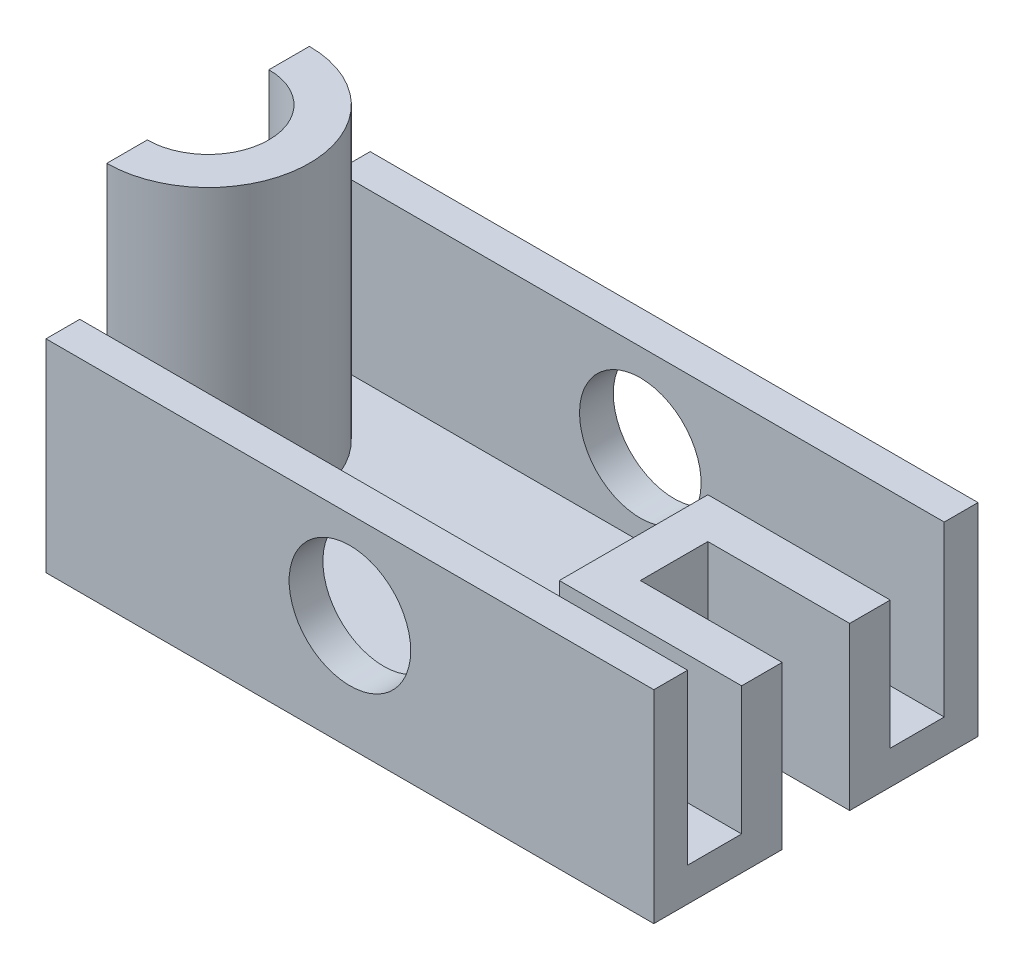
ISO-10303-21;
HEADER;
FILE_DESCRIPTION(('STEP AP214'),'2;1');
FILE_NAME('part.step','',(''),(''),'','','');
FILE_SCHEMA(('AUTOMOTIVE_DESIGN { 1 0 10303 214 1 1 1 1 }'));
ENDSEC;
DATA;
#1=APPLICATION_CONTEXT('core data for automotive mechanical design processes');
#2=APPLICATION_PROTOCOL_DEFINITION('international standard','automotive_design',2000,#1);
#3=PRODUCT_CONTEXT('',#1,'mechanical');
#4=PRODUCT('Part','Part','',(#3));
#5=PRODUCT_RELATED_PRODUCT_CATEGORY('part','',(#4));
#6=PRODUCT_DEFINITION_FORMATION('','',#4);
#7=PRODUCT_DEFINITION_CONTEXT('part definition',#1,'design');
#8=PRODUCT_DEFINITION('design','',#6,#7);
#9=PRODUCT_DEFINITION_SHAPE('','',#8);
#10=(LENGTH_UNIT() NAMED_UNIT(*) SI_UNIT(.MILLI.,.METRE.));
#11=(NAMED_UNIT(*) PLANE_ANGLE_UNIT() SI_UNIT($,.RADIAN.));
#12=(NAMED_UNIT(*) SI_UNIT($,.STERADIAN.) SOLID_ANGLE_UNIT());
#13=UNCERTAINTY_MEASURE_WITH_UNIT(LENGTH_MEASURE(1.E-05),#10,'distance_accuracy_value','');
#14=(GEOMETRIC_REPRESENTATION_CONTEXT(3) GLOBAL_UNCERTAINTY_ASSIGNED_CONTEXT((#13)) GLOBAL_UNIT_ASSIGNED_CONTEXT((#10,
#11,#12)) REPRESENTATION_CONTEXT('',''));
#15=CARTESIAN_POINT('',(0.,0.,0.));
#16=DIRECTION('',(0.,0.,1.));
#17=DIRECTION('',(1.,0.,0.));
#18=AXIS2_PLACEMENT_3D('',#15,#16,#17);
#19=CARTESIAN_POINT('',(45.,30.,24.));
#20=DIRECTION('',(-1.,0.,0.));
#21=DIRECTION('',(0.,0.,1.));
#22=AXIS2_PLACEMENT_3D('',#19,#20,#21);
#23=PLANE('',#22);
#24=DIRECTION('',(0.,0.,-1.));
#25=VECTOR('',#24,1.);
#26=CARTESIAN_POINT('',(45.,0.,24.));
#27=LINE('',#26,#25);
#28=CARTESIAN_POINT('',(45.,0.,24.));
#29=VERTEX_POINT('',#28);
#30=CARTESIAN_POINT('',(45.,0.,5.));
#31=VERTEX_POINT('',#30);
#32=EDGE_CURVE('E202',#29,#31,#27,.T.);
#33=ORIENTED_EDGE('',*,*,#32,.T.);
#34=DIRECTION('',(0.,1.,0.));
#35=VECTOR('',#34,1.);
#36=CARTESIAN_POINT('',(45.,0.,5.));
#37=LINE('',#36,#35);
#38=CARTESIAN_POINT('',(45.,24.,5.));
#39=VERTEX_POINT('',#38);
#40=EDGE_CURVE('E251',#31,#39,#37,.T.);
#41=ORIENTED_EDGE('',*,*,#40,.T.);
#42=DIRECTION('',(0.,0.,-1.));
#43=VECTOR('',#42,1.);
#44=CARTESIAN_POINT('',(45.,24.,-11.));
#45=LINE('',#44,#43);
#46=CARTESIAN_POINT('',(45.,24.,11.));
#47=VERTEX_POINT('',#46);
#48=EDGE_CURVE('E257',#47,#39,#45,.T.);
#49=ORIENTED_EDGE('',*,*,#48,.F.);
#50=DIRECTION('',(0.,-1.,0.));
#51=VECTOR('',#50,1.);
#52=CARTESIAN_POINT('',(45.,24.,11.));
#53=LINE('',#52,#51);
#54=CARTESIAN_POINT('',(45.,5.,11.));
#55=VERTEX_POINT('',#54);
#56=EDGE_CURVE('E267',#47,#55,#53,.T.);
#57=ORIENTED_EDGE('',*,*,#56,.T.);
#58=DIRECTION('',(0.,0.,1.));
#59=VECTOR('',#58,1.);
#60=CARTESIAN_POINT('',(45.,5.,-19.));
#61=LINE('',#60,#59);
#62=CARTESIAN_POINT('',(45.,5.,19.));
#63=VERTEX_POINT('',#62);
#64=EDGE_CURVE('E314',#55,#63,#61,.T.);
#65=ORIENTED_EDGE('',*,*,#64,.T.);
#66=DIRECTION('',(0.,1.,0.));
#67=VECTOR('',#66,1.);
#68=CARTESIAN_POINT('',(45.,30.,19.));
#69=LINE('',#68,#67);
#70=CARTESIAN_POINT('',(45.,30.,19.));
#71=VERTEX_POINT('',#70);
#72=EDGE_CURVE('E317',#63,#71,#69,.T.);
#73=ORIENTED_EDGE('',*,*,#72,.T.);
#74=DIRECTION('',(0.,0.,-1.));
#75=VECTOR('',#74,1.);
#76=CARTESIAN_POINT('',(45.,30.,24.));
#77=LINE('',#76,#75);
#78=CARTESIAN_POINT('',(45.,30.,24.));
#79=VERTEX_POINT('',#78);
#80=EDGE_CURVE('E333',#79,#71,#77,.T.);
#81=ORIENTED_EDGE('',*,*,#80,.F.);
#82=DIRECTION('',(0.,-1.,0.));
#83=VECTOR('',#82,1.);
#84=CARTESIAN_POINT('',(45.,30.,24.));
#85=LINE('',#84,#83);
#86=EDGE_CURVE('E224',#79,#29,#85,.T.);
#87=ORIENTED_EDGE('',*,*,#86,.T.);
#88=EDGE_LOOP('',(#33,#41,#49,#57,#65,#73,#81,#87));
#89=FACE_BOUND('',#88,.T.);
#90=ADVANCED_FACE('F43',(#89),#23,.F.);
#91=CARTESIAN_POINT('',(45.,5.,-19.));
#92=DIRECTION('',(0.,-1.,0.));
#93=DIRECTION('',(0.,0.,-1.));
#94=AXIS2_PLACEMENT_3D('',#91,#92,#93);
#95=PLANE('',#94);
#96=DIRECTION('',(-1.,0.,0.));
#97=VECTOR('',#96,1.);
#98=CARTESIAN_POINT('',(45.,5.,-11.));
#99=LINE('',#98,#97);
#100=CARTESIAN_POINT('',(45.,5.,-11.));
#101=VERTEX_POINT('',#100);
#102=CARTESIAN_POINT('',(18.,5.,-11.));
#103=VERTEX_POINT('',#102);
#104=EDGE_CURVE('E258',#101,#103,#99,.T.);
#105=ORIENTED_EDGE('',*,*,#104,.F.);
#106=CARTESIAN_POINT('',(45.,5.,-19.));
#107=VERTEX_POINT('',#106);
#108=EDGE_CURVE('E316',#107,#101,#61,.T.);
#109=ORIENTED_EDGE('',*,*,#108,.F.);
#110=DIRECTION('',(-1.,0.,0.));
#111=VECTOR('',#110,1.);
#112=CARTESIAN_POINT('',(45.,5.,-19.));
#113=LINE('',#112,#111);
#114=CARTESIAN_POINT('',(-45.,5.,-19.));
#115=VERTEX_POINT('',#114);
#116=EDGE_CURVE('E325',#107,#115,#113,.T.);
#117=ORIENTED_EDGE('',*,*,#116,.T.);
#118=DIRECTION('',(0.,0.,1.));
#119=VECTOR('',#118,1.);
#120=CARTESIAN_POINT('',(-45.,5.,-19.));
#121=LINE('',#120,#119);
#122=CARTESIAN_POINT('',(-45.,5.,-15.));
#123=VERTEX_POINT('',#122);
#124=EDGE_CURVE('E326',#115,#123,#121,.T.);
#125=ORIENTED_EDGE('',*,*,#124,.T.);
#126=CARTESIAN_POINT('',(-45.,5.,0.));
#127=DIRECTION('',(0.,-1.,0.));
#128=DIRECTION('',(0.,0.,-1.));
#129=AXIS2_PLACEMENT_3D('',#126,#127,#128);
#130=CIRCLE('',#129,15.);
#131=CARTESIAN_POINT('',(-45.,5.,15.));
#132=VERTEX_POINT('',#131);
#133=EDGE_CURVE('E11',#123,#132,#130,.T.);
#134=ORIENTED_EDGE('',*,*,#133,.T.);
#135=CARTESIAN_POINT('',(-45.,5.,19.));
#136=VERTEX_POINT('',#135);
#137=EDGE_CURVE('E324',#132,#136,#121,.T.);
#138=ORIENTED_EDGE('',*,*,#137,.T.);
#139=DIRECTION('',(-1.,0.,0.));
#140=VECTOR('',#139,1.);
#141=CARTESIAN_POINT('',(45.,5.,19.));
#142=LINE('',#141,#140);
#143=EDGE_CURVE('E332',#63,#136,#142,.T.);
#144=ORIENTED_EDGE('',*,*,#143,.F.);
#145=ORIENTED_EDGE('',*,*,#64,.F.);
#146=DIRECTION('',(1.,0.,0.));
#147=VECTOR('',#146,1.);
#148=CARTESIAN_POINT('',(45.,5.,11.));
#149=LINE('',#148,#147);
#150=CARTESIAN_POINT('',(18.,5.,11.));
#151=VERTEX_POINT('',#150);
#152=EDGE_CURVE('E275',#151,#55,#149,.T.);
#153=ORIENTED_EDGE('',*,*,#152,.F.);
#154=DIRECTION('',(0.,0.,1.));
#155=VECTOR('',#154,1.);
#156=CARTESIAN_POINT('',(18.,5.,-11.));
#157=LINE('',#156,#155);
#158=EDGE_CURVE('E66',#103,#151,#157,.T.);
#159=ORIENTED_EDGE('',*,*,#158,.F.);
#160=EDGE_LOOP('',(#105,#109,#117,#125,#134,#138,#144,#145,#153,#159));
#161=FACE_BOUND('',#160,.T.);
#162=ADVANCED_FACE('F368',(#161),#95,.F.);
#163=CARTESIAN_POINT('',(-45.,30.,24.));
#164=DIRECTION('',(1.,0.,0.));
#165=DIRECTION('',(0.,0.,-1.));
#166=AXIS2_PLACEMENT_3D('',#163,#164,#165);
#167=PLANE('',#166);
#168=DIRECTION('',(0.,0.,1.));
#169=VECTOR('',#168,1.);
#170=CARTESIAN_POINT('',(-45.,0.,24.));
#171=LINE('',#170,#169);
#172=CARTESIAN_POINT('',(-45.,0.,-24.));
#173=VERTEX_POINT('',#172);
#174=CARTESIAN_POINT('',(-45.,0.,-9.00000000000001));
#175=VERTEX_POINT('',#174);
#176=EDGE_CURVE('E220',#173,#175,#171,.T.);
#177=ORIENTED_EDGE('',*,*,#176,.T.);
#178=DIRECTION('',(0.,1.,0.));
#179=VECTOR('',#178,1.);
#180=CARTESIAN_POINT('',(-45.,0.,-9.00000000000001));
#181=LINE('',#180,#179);
#182=CARTESIAN_POINT('',(-45.,48.,-9.00000000000001));
#183=VERTEX_POINT('',#182);
#184=EDGE_CURVE('E294',#175,#183,#181,.T.);
#185=ORIENTED_EDGE('',*,*,#184,.T.);
#186=DIRECTION('',(0.,0.,-1.));
#187=VECTOR('',#186,1.);
#188=CARTESIAN_POINT('',(-45.,48.,15.));
#189=LINE('',#188,#187);
#190=CARTESIAN_POINT('',(-45.,48.,-15.));
#191=VERTEX_POINT('',#190);
#192=EDGE_CURVE('E300',#183,#191,#189,.T.);
#193=ORIENTED_EDGE('',*,*,#192,.T.);
#194=DIRECTION('',(0.,-1.,0.));
#195=VECTOR('',#194,1.);
#196=CARTESIAN_POINT('',(-45.,48.,-15.));
#197=LINE('',#196,#195);
#198=EDGE_CURVE('E304',#191,#123,#197,.T.);
#199=ORIENTED_EDGE('',*,*,#198,.T.);
#200=ORIENTED_EDGE('',*,*,#124,.F.);
#201=DIRECTION('',(0.,-1.,0.));
#202=VECTOR('',#201,1.);
#203=CARTESIAN_POINT('',(-45.,30.,-19.));
#204=LINE('',#203,#202);
#205=CARTESIAN_POINT('',(-45.,30.,-19.));
#206=VERTEX_POINT('',#205);
#207=EDGE_CURVE('E306',#206,#115,#204,.T.);
#208=ORIENTED_EDGE('',*,*,#207,.F.);
#209=DIRECTION('',(0.,0.,1.));
#210=VECTOR('',#209,1.);
#211=CARTESIAN_POINT('',(-45.,30.,24.));
#212=LINE('',#211,#210);
#213=CARTESIAN_POINT('',(-45.,30.,-24.));
#214=VERTEX_POINT('',#213);
#215=EDGE_CURVE('E340',#214,#206,#212,.T.);
#216=ORIENTED_EDGE('',*,*,#215,.F.);
#217=DIRECTION('',(0.,-1.,0.));
#218=VECTOR('',#217,1.);
#219=CARTESIAN_POINT('',(-45.,30.,-24.));
#220=LINE('',#219,#218);
#221=EDGE_CURVE('E228',#214,#173,#220,.T.);
#222=ORIENTED_EDGE('',*,*,#221,.T.);
#223=EDGE_LOOP('',(#177,#185,#193,#199,#200,#208,#216,#222));
#224=FACE_BOUND('',#223,.T.);
#225=ADVANCED_FACE('F409',(#224),#167,.F.);
#226=CARTESIAN_POINT('',(0.,30.,0.));
#227=DIRECTION('',(0.,-1.,0.));
#228=DIRECTION('',(0.,0.,-1.));
#229=AXIS2_PLACEMENT_3D('',#226,#227,#228);
#230=PLANE('',#229);
#231=ORIENTED_EDGE('',*,*,#215,.T.);
#232=DIRECTION('',(-1.,0.,0.));
#233=VECTOR('',#232,1.);
#234=CARTESIAN_POINT('',(45.,30.,-19.));
#235=LINE('',#234,#233);
#236=CARTESIAN_POINT('',(45.,30.,-19.));
#237=VERTEX_POINT('',#236);
#238=EDGE_CURVE('E206',#237,#206,#235,.T.);
#239=ORIENTED_EDGE('',*,*,#238,.F.);
#240=CARTESIAN_POINT('',(45.,30.,-24.));
#241=VERTEX_POINT('',#240);
#242=EDGE_CURVE('E225',#237,#241,#77,.T.);
#243=ORIENTED_EDGE('',*,*,#242,.T.);
#244=DIRECTION('',(-1.,0.,0.));
#245=VECTOR('',#244,1.);
#246=CARTESIAN_POINT('',(-45.,30.,-24.));
#247=LINE('',#246,#245);
#248=EDGE_CURVE('E339',#241,#214,#247,.T.);
#249=ORIENTED_EDGE('',*,*,#248,.T.);
#250=EDGE_LOOP('',(#231,#239,#243,#249));
#251=FACE_BOUND('',#250,.T.);
#252=ADVANCED_FACE('F405',(#251),#230,.F.);
#253=CARTESIAN_POINT('',(45.,24.,-5.));
#254=VERTEX_POINT('',#253);
#255=CARTESIAN_POINT('',(45.,24.,-11.));
#256=VERTEX_POINT('',#255);
#257=EDGE_CURVE('E197',#254,#256,#45,.T.);
#258=ORIENTED_EDGE('',*,*,#257,.F.);
#259=DIRECTION('',(0.,1.,0.));
#260=VECTOR('',#259,1.);
#261=CARTESIAN_POINT('',(45.,0.,-5.));
#262=LINE('',#261,#260);
#263=CARTESIAN_POINT('',(45.,0.,-5.));
#264=VERTEX_POINT('',#263);
#265=EDGE_CURVE('E58',#264,#254,#262,.T.);
#266=ORIENTED_EDGE('',*,*,#265,.F.);
#267=CARTESIAN_POINT('',(45.,0.,-24.));
#268=VERTEX_POINT('',#267);
#269=EDGE_CURVE('E192',#264,#268,#27,.T.);
#270=ORIENTED_EDGE('',*,*,#269,.T.);
#271=DIRECTION('',(0.,-1.,0.));
#272=VECTOR('',#271,1.);
#273=CARTESIAN_POINT('',(45.,30.,-24.));
#274=LINE('',#273,#272);
#275=EDGE_CURVE('E55',#241,#268,#274,.T.);
#276=ORIENTED_EDGE('',*,*,#275,.F.);
#277=ORIENTED_EDGE('',*,*,#242,.F.);
#278=DIRECTION('',(0.,-1.,0.));
#279=VECTOR('',#278,1.);
#280=CARTESIAN_POINT('',(45.,30.,-19.));
#281=LINE('',#280,#279);
#282=EDGE_CURVE('E313',#237,#107,#281,.T.);
#283=ORIENTED_EDGE('',*,*,#282,.T.);
#284=ORIENTED_EDGE('',*,*,#108,.T.);
#285=DIRECTION('',(0.,-1.,0.));
#286=VECTOR('',#285,1.);
#287=CARTESIAN_POINT('',(45.,24.,-11.));
#288=LINE('',#287,#286);
#289=EDGE_CURVE('E284',#256,#101,#288,.T.);
#290=ORIENTED_EDGE('',*,*,#289,.F.);
#291=EDGE_LOOP('',(#258,#266,#270,#276,#277,#283,#284,#290));
#292=FACE_BOUND('',#291,.T.);
#293=ADVANCED_FACE('F44',(#292),#23,.F.);
#294=CARTESIAN_POINT('',(-45.,30.,-24.));
#295=DIRECTION('',(0.,0.,1.));
#296=DIRECTION('',(1.,0.,0.));
#297=AXIS2_PLACEMENT_3D('',#294,#295,#296);
#298=PLANE('',#297);
#299=CARTESIAN_POINT('',(0.,17.,-24.));
#300=DIRECTION('',(0.,0.,-1.));
#301=DIRECTION('',(-1.,0.,0.));
#302=AXIS2_PLACEMENT_3D('',#299,#300,#301);
#303=CIRCLE('',#302,9.);
#304=CARTESIAN_POINT('',(-9.,17.,-24.));
#305=VERTEX_POINT('',#304);
#306=EDGE_CURVE('E245',#305,#305,#303,.T.);
#307=ORIENTED_EDGE('',*,*,#306,.F.);
#308=EDGE_LOOP('',(#307));
#309=FACE_BOUND('',#308,.T.);
#310=DIRECTION('',(-1.,0.,0.));
#311=VECTOR('',#310,1.);
#312=CARTESIAN_POINT('',(-45.,0.,-24.));
#313=LINE('',#312,#311);
#314=EDGE_CURVE('E201',#268,#173,#313,.T.);
#315=ORIENTED_EDGE('',*,*,#314,.T.);
#316=ORIENTED_EDGE('',*,*,#221,.F.);
#317=ORIENTED_EDGE('',*,*,#248,.F.);
#318=ORIENTED_EDGE('',*,*,#275,.T.);
#319=EDGE_LOOP('',(#315,#316,#317,#318));
#320=FACE_BOUND('',#319,.T.);
#321=ADVANCED_FACE('F406',(#309,#320),#298,.F.);
#322=CARTESIAN_POINT('',(-45.,48.,15.));
#323=VERTEX_POINT('',#322);
#324=CARTESIAN_POINT('',(-45.,48.,9.));
#325=VERTEX_POINT('',#324);
#326=EDGE_CURVE('E303',#323,#325,#189,.T.);
#327=ORIENTED_EDGE('',*,*,#326,.T.);
#328=DIRECTION('',(0.,1.,0.));
#329=VECTOR('',#328,1.);
#330=CARTESIAN_POINT('',(-45.,0.,9.));
#331=LINE('',#330,#329);
#332=CARTESIAN_POINT('',(-45.,0.,9.));
#333=VERTEX_POINT('',#332);
#334=EDGE_CURVE('E289',#325,#333,#331,.F.);
#335=ORIENTED_EDGE('',*,*,#334,.T.);
#336=CARTESIAN_POINT('',(-45.,0.,24.));
#337=VERTEX_POINT('',#336);
#338=EDGE_CURVE('E216',#333,#337,#171,.T.);
#339=ORIENTED_EDGE('',*,*,#338,.T.);
#340=DIRECTION('',(0.,-1.,0.));
#341=VECTOR('',#340,1.);
#342=CARTESIAN_POINT('',(-45.,30.,24.));
#343=LINE('',#342,#341);
#344=CARTESIAN_POINT('',(-45.,30.,24.));
#345=VERTEX_POINT('',#344);
#346=EDGE_CURVE('E226',#345,#337,#343,.T.);
#347=ORIENTED_EDGE('',*,*,#346,.F.);
#348=CARTESIAN_POINT('',(-45.,30.,19.));
#349=VERTEX_POINT('',#348);
#350=EDGE_CURVE('E338',#349,#345,#212,.T.);
#351=ORIENTED_EDGE('',*,*,#350,.F.);
#352=DIRECTION('',(0.,1.,0.));
#353=VECTOR('',#352,1.);
#354=CARTESIAN_POINT('',(-45.,30.,19.));
#355=LINE('',#354,#353);
#356=EDGE_CURVE('E312',#136,#349,#355,.T.);
#357=ORIENTED_EDGE('',*,*,#356,.F.);
#358=ORIENTED_EDGE('',*,*,#137,.F.);
#359=DIRECTION('',(0.,-1.,0.));
#360=VECTOR('',#359,1.);
#361=CARTESIAN_POINT('',(-45.,48.,15.));
#362=LINE('',#361,#360);
#363=EDGE_CURVE('E302',#323,#132,#362,.T.);
#364=ORIENTED_EDGE('',*,*,#363,.F.);
#365=EDGE_LOOP('',(#327,#335,#339,#347,#351,#357,#358,#364));
#366=FACE_BOUND('',#365,.T.);
#367=ADVANCED_FACE('F354',(#366),#167,.F.);
#368=CARTESIAN_POINT('',(-45.,30.,24.));
#369=DIRECTION('',(0.,0.,-1.));
#370=DIRECTION('',(-1.,0.,0.));
#371=AXIS2_PLACEMENT_3D('',#368,#369,#370);
#372=PLANE('',#371);
#373=CARTESIAN_POINT('',(0.,17.,24.));
#374=DIRECTION('',(0.,0.,1.));
#375=DIRECTION('',(1.,0.,0.));
#376=AXIS2_PLACEMENT_3D('',#373,#374,#375);
#377=CIRCLE('',#376,9.);
#378=CARTESIAN_POINT('',(9.,17.,24.));
#379=VERTEX_POINT('',#378);
#380=EDGE_CURVE('E234',#379,#379,#377,.T.);
#381=ORIENTED_EDGE('',*,*,#380,.F.);
#382=EDGE_LOOP('',(#381));
#383=FACE_BOUND('',#382,.T.);
#384=DIRECTION('',(1.,0.,0.));
#385=VECTOR('',#384,1.);
#386=CARTESIAN_POINT('',(-45.,0.,24.));
#387=LINE('',#386,#385);
#388=EDGE_CURVE('E219',#337,#29,#387,.T.);
#389=ORIENTED_EDGE('',*,*,#388,.T.);
#390=ORIENTED_EDGE('',*,*,#86,.F.);
#391=DIRECTION('',(1.,0.,0.));
#392=VECTOR('',#391,1.);
#393=CARTESIAN_POINT('',(-45.,30.,24.));
#394=LINE('',#393,#392);
#395=EDGE_CURVE('E213',#345,#79,#394,.T.);
#396=ORIENTED_EDGE('',*,*,#395,.F.);
#397=ORIENTED_EDGE('',*,*,#346,.T.);
#398=EDGE_LOOP('',(#389,#390,#396,#397));
#399=FACE_BOUND('',#398,.T.);
#400=ADVANCED_FACE('F360',(#383,#399),#372,.F.);
#401=ORIENTED_EDGE('',*,*,#80,.T.);
#402=DIRECTION('',(-1.,0.,0.));
#403=VECTOR('',#402,1.);
#404=CARTESIAN_POINT('',(45.,30.,19.));
#405=LINE('',#404,#403);
#406=EDGE_CURVE('E207',#71,#349,#405,.T.);
#407=ORIENTED_EDGE('',*,*,#406,.T.);
#408=ORIENTED_EDGE('',*,*,#350,.T.);
#409=ORIENTED_EDGE('',*,*,#395,.T.);
#410=EDGE_LOOP('',(#401,#407,#408,#409));
#411=FACE_BOUND('',#410,.T.);
#412=ADVANCED_FACE('F346',(#411),#230,.F.);
#413=CARTESIAN_POINT('',(0.,0.,0.));
#414=DIRECTION('',(0.,-1.,0.));
#415=DIRECTION('',(0.,0.,-1.));
#416=AXIS2_PLACEMENT_3D('',#413,#414,#415);
#417=PLANE('',#416);
#418=DIRECTION('',(1.,0.,0.));
#419=VECTOR('',#418,1.);
#420=CARTESIAN_POINT('',(45.,0.,5.));
#421=LINE('',#420,#419);
#422=CARTESIAN_POINT('',(24.,0.,5.));
#423=VERTEX_POINT('',#422);
#424=EDGE_CURVE('E196',#423,#31,#421,.T.);
#425=ORIENTED_EDGE('',*,*,#424,.T.);
#426=ORIENTED_EDGE('',*,*,#32,.F.);
#427=ORIENTED_EDGE('',*,*,#388,.F.);
#428=ORIENTED_EDGE('',*,*,#338,.F.);
#429=CARTESIAN_POINT('',(-45.,0.,0.));
#430=DIRECTION('',(0.,1.,0.));
#431=DIRECTION('',(0.,0.,1.));
#432=AXIS2_PLACEMENT_3D('',#429,#430,#431);
#433=CIRCLE('',#432,9.);
#434=EDGE_CURVE('E290',#333,#175,#433,.T.);
#435=ORIENTED_EDGE('',*,*,#434,.T.);
#436=ORIENTED_EDGE('',*,*,#176,.F.);
#437=ORIENTED_EDGE('',*,*,#314,.F.);
#438=ORIENTED_EDGE('',*,*,#269,.F.);
#439=DIRECTION('',(-1.,0.,0.));
#440=VECTOR('',#439,1.);
#441=CARTESIAN_POINT('',(45.,0.,-5.));
#442=LINE('',#441,#440);
#443=CARTESIAN_POINT('',(24.,0.,-5.));
#444=VERTEX_POINT('',#443);
#445=EDGE_CURVE('E182',#264,#444,#442,.T.);
#446=ORIENTED_EDGE('',*,*,#445,.T.);
#447=DIRECTION('',(0.,0.,1.));
#448=VECTOR('',#447,1.);
#449=CARTESIAN_POINT('',(24.,0.,-5.));
#450=LINE('',#449,#448);
#451=EDGE_CURVE('E189',#444,#423,#450,.T.);
#452=ORIENTED_EDGE('',*,*,#451,.T.);
#453=EDGE_LOOP('',(#425,#426,#427,#428,#435,#436,#437,#438,#446,#452));
#454=FACE_BOUND('',#453,.T.);
#455=ADVANCED_FACE('F203',(#454),#417,.T.);
#456=CARTESIAN_POINT('',(45.,30.,-19.));
#457=DIRECTION('',(0.,0.,-1.));
#458=DIRECTION('',(0.,1.,0.));
#459=AXIS2_PLACEMENT_3D('',#456,#457,#458);
#460=PLANE('',#459);
#461=CARTESIAN_POINT('',(0.,17.,-19.));
#462=DIRECTION('',(0.,0.,-1.));
#463=DIRECTION('',(0.,1.,0.));
#464=AXIS2_PLACEMENT_3D('',#461,#462,#463);
#465=CIRCLE('',#464,9.);
#466=CARTESIAN_POINT('',(0.,26.,-19.));
#467=VERTEX_POINT('',#466);
#468=EDGE_CURVE('E50',#467,#467,#465,.T.);
#469=ORIENTED_EDGE('',*,*,#468,.T.);
#470=EDGE_LOOP('',(#469));
#471=FACE_BOUND('',#470,.T.);
#472=ORIENTED_EDGE('',*,*,#207,.T.);
#473=ORIENTED_EDGE('',*,*,#116,.F.);
#474=ORIENTED_EDGE('',*,*,#282,.F.);
#475=ORIENTED_EDGE('',*,*,#238,.T.);
#476=EDGE_LOOP('',(#472,#473,#474,#475));
#477=FACE_BOUND('',#476,.T.);
#478=ADVANCED_FACE('F399',(#471,#477),#460,.F.);
#479=CARTESIAN_POINT('',(45.,30.,19.));
#480=DIRECTION('',(0.,0.,1.));
#481=DIRECTION('',(0.,-1.,0.));
#482=AXIS2_PLACEMENT_3D('',#479,#480,#481);
#483=PLANE('',#482);
#484=CARTESIAN_POINT('',(0.,17.,19.));
#485=DIRECTION('',(0.,0.,1.));
#486=DIRECTION('',(0.,-1.,0.));
#487=AXIS2_PLACEMENT_3D('',#484,#485,#486);
#488=CIRCLE('',#487,9.);
#489=CARTESIAN_POINT('',(0.,8.,19.));
#490=VERTEX_POINT('',#489);
#491=EDGE_CURVE('E235',#490,#490,#488,.T.);
#492=ORIENTED_EDGE('',*,*,#491,.T.);
#493=EDGE_LOOP('',(#492));
#494=FACE_BOUND('',#493,.T.);
#495=ORIENTED_EDGE('',*,*,#356,.T.);
#496=ORIENTED_EDGE('',*,*,#406,.F.);
#497=ORIENTED_EDGE('',*,*,#72,.F.);
#498=ORIENTED_EDGE('',*,*,#143,.T.);
#499=EDGE_LOOP('',(#495,#496,#497,#498));
#500=FACE_BOUND('',#499,.T.);
#501=ADVANCED_FACE('F365',(#494,#500),#483,.F.);
#502=CARTESIAN_POINT('',(-45.,48.,0.));
#503=DIRECTION('',(0.,-1.,0.));
#504=DIRECTION('',(0.,0.,-1.));
#505=AXIS2_PLACEMENT_3D('',#502,#503,#504);
#506=CYLINDRICAL_SURFACE('',#505,15.);
#507=ORIENTED_EDGE('',*,*,#133,.F.);
#508=ORIENTED_EDGE('',*,*,#198,.F.);
#509=CARTESIAN_POINT('',(-45.,48.,0.));
#510=DIRECTION('',(0.,-1.,0.));
#511=DIRECTION('',(0.,0.,-1.));
#512=AXIS2_PLACEMENT_3D('',#509,#510,#511);
#513=CIRCLE('',#512,15.);
#514=EDGE_CURVE('E297',#191,#323,#513,.T.);
#515=ORIENTED_EDGE('',*,*,#514,.T.);
#516=ORIENTED_EDGE('',*,*,#363,.T.);
#517=EDGE_LOOP('',(#507,#508,#515,#516));
#518=FACE_BOUND('',#517,.T.);
#519=ADVANCED_FACE('F367',(#518),#506,.T.);
#520=CARTESIAN_POINT('',(-45.,48.,0.));
#521=DIRECTION('',(0.,-1.,0.));
#522=DIRECTION('',(0.,0.,-1.));
#523=AXIS2_PLACEMENT_3D('',#520,#521,#522);
#524=PLANE('',#523);
#525=ORIENTED_EDGE('',*,*,#192,.F.);
#526=CARTESIAN_POINT('',(-45.,48.,0.));
#527=DIRECTION('',(0.,1.,0.));
#528=DIRECTION('',(0.,0.,1.));
#529=AXIS2_PLACEMENT_3D('',#526,#527,#528);
#530=CIRCLE('',#529,9.);
#531=EDGE_CURVE('E288',#325,#183,#530,.T.);
#532=ORIENTED_EDGE('',*,*,#531,.F.);
#533=ORIENTED_EDGE('',*,*,#326,.F.);
#534=ORIENTED_EDGE('',*,*,#514,.F.);
#535=EDGE_LOOP('',(#525,#532,#533,#534));
#536=FACE_BOUND('',#535,.T.);
#537=ADVANCED_FACE('F376',(#536),#524,.F.);
#538=CARTESIAN_POINT('',(-45.,0.,0.));
#539=DIRECTION('',(0.,1.,0.));
#540=DIRECTION('',(0.,0.,1.));
#541=AXIS2_PLACEMENT_3D('',#538,#539,#540);
#542=CYLINDRICAL_SURFACE('',#541,9.);
#543=ORIENTED_EDGE('',*,*,#434,.F.);
#544=ORIENTED_EDGE('',*,*,#334,.F.);
#545=ORIENTED_EDGE('',*,*,#531,.T.);
#546=ORIENTED_EDGE('',*,*,#184,.F.);
#547=EDGE_LOOP('',(#543,#544,#545,#546));
#548=FACE_BOUND('',#547,.T.);
#549=ADVANCED_FACE('F408',(#548),#542,.F.);
#550=CARTESIAN_POINT('',(45.,24.,-11.));
#551=DIRECTION('',(0.,0.,1.));
#552=DIRECTION('',(1.,0.,0.));
#553=AXIS2_PLACEMENT_3D('',#550,#551,#552);
#554=PLANE('',#553);
#555=ORIENTED_EDGE('',*,*,#104,.T.);
#556=DIRECTION('',(0.,-1.,0.));
#557=VECTOR('',#556,1.);
#558=CARTESIAN_POINT('',(18.,24.,-11.));
#559=LINE('',#558,#557);
#560=CARTESIAN_POINT('',(18.,24.,-11.));
#561=VERTEX_POINT('',#560);
#562=EDGE_CURVE('E278',#561,#103,#559,.T.);
#563=ORIENTED_EDGE('',*,*,#562,.F.);
#564=DIRECTION('',(-1.,0.,0.));
#565=VECTOR('',#564,1.);
#566=CARTESIAN_POINT('',(45.,24.,-11.));
#567=LINE('',#566,#565);
#568=EDGE_CURVE('E263',#256,#561,#567,.T.);
#569=ORIENTED_EDGE('',*,*,#568,.F.);
#570=ORIENTED_EDGE('',*,*,#289,.T.);
#571=EDGE_LOOP('',(#555,#563,#569,#570));
#572=FACE_BOUND('',#571,.T.);
#573=ADVANCED_FACE('F398',(#572),#554,.F.);
#574=CARTESIAN_POINT('',(18.,24.,-11.));
#575=DIRECTION('',(1.,0.,0.));
#576=DIRECTION('',(0.,0.,-1.));
#577=AXIS2_PLACEMENT_3D('',#574,#575,#576);
#578=PLANE('',#577);
#579=ORIENTED_EDGE('',*,*,#158,.T.);
#580=DIRECTION('',(0.,-1.,0.));
#581=VECTOR('',#580,1.);
#582=CARTESIAN_POINT('',(18.,24.,11.));
#583=LINE('',#582,#581);
#584=CARTESIAN_POINT('',(18.,24.,11.));
#585=VERTEX_POINT('',#584);
#586=EDGE_CURVE('E280',#585,#151,#583,.T.);
#587=ORIENTED_EDGE('',*,*,#586,.F.);
#588=DIRECTION('',(0.,0.,1.));
#589=VECTOR('',#588,1.);
#590=CARTESIAN_POINT('',(18.,24.,-11.));
#591=LINE('',#590,#589);
#592=EDGE_CURVE('E264',#561,#585,#591,.T.);
#593=ORIENTED_EDGE('',*,*,#592,.F.);
#594=ORIENTED_EDGE('',*,*,#562,.T.);
#595=EDGE_LOOP('',(#579,#587,#593,#594));
#596=FACE_BOUND('',#595,.T.);
#597=ADVANCED_FACE('F392',(#596),#578,.F.);
#598=CARTESIAN_POINT('',(45.,24.,11.));
#599=DIRECTION('',(0.,0.,-1.));
#600=DIRECTION('',(-1.,0.,0.));
#601=AXIS2_PLACEMENT_3D('',#598,#599,#600);
#602=PLANE('',#601);
#603=ORIENTED_EDGE('',*,*,#152,.T.);
#604=ORIENTED_EDGE('',*,*,#56,.F.);
#605=DIRECTION('',(1.,0.,0.));
#606=VECTOR('',#605,1.);
#607=CARTESIAN_POINT('',(45.,24.,11.));
#608=LINE('',#607,#606);
#609=EDGE_CURVE('E270',#585,#47,#608,.T.);
#610=ORIENTED_EDGE('',*,*,#609,.F.);
#611=ORIENTED_EDGE('',*,*,#586,.T.);
#612=EDGE_LOOP('',(#603,#604,#610,#611));
#613=FACE_BOUND('',#612,.T.);
#614=ADVANCED_FACE('F388',(#613),#602,.F.);
#615=CARTESIAN_POINT('',(0.,24.,0.));
#616=DIRECTION('',(0.,-1.,0.));
#617=DIRECTION('',(0.,0.,-1.));
#618=AXIS2_PLACEMENT_3D('',#615,#616,#617);
#619=PLANE('',#618);
#620=ORIENTED_EDGE('',*,*,#48,.T.);
#621=DIRECTION('',(1.,0.,0.));
#622=VECTOR('',#621,1.);
#623=CARTESIAN_POINT('',(45.,24.,5.));
#624=LINE('',#623,#622);
#625=CARTESIAN_POINT('',(24.,24.,5.));
#626=VERTEX_POINT('',#625);
#627=EDGE_CURVE('E188',#626,#39,#624,.T.);
#628=ORIENTED_EDGE('',*,*,#627,.F.);
#629=DIRECTION('',(0.,0.,1.));
#630=VECTOR('',#629,1.);
#631=CARTESIAN_POINT('',(24.,24.,-5.));
#632=LINE('',#631,#630);
#633=CARTESIAN_POINT('',(24.,24.,-5.));
#634=VERTEX_POINT('',#633);
#635=EDGE_CURVE('E236',#634,#626,#632,.T.);
#636=ORIENTED_EDGE('',*,*,#635,.F.);
#637=DIRECTION('',(-1.,0.,0.));
#638=VECTOR('',#637,1.);
#639=CARTESIAN_POINT('',(45.,24.,-5.));
#640=LINE('',#639,#638);
#641=EDGE_CURVE('E232',#254,#634,#640,.T.);
#642=ORIENTED_EDGE('',*,*,#641,.F.);
#643=ORIENTED_EDGE('',*,*,#257,.T.);
#644=ORIENTED_EDGE('',*,*,#568,.T.);
#645=ORIENTED_EDGE('',*,*,#592,.T.);
#646=ORIENTED_EDGE('',*,*,#609,.T.);
#647=EDGE_LOOP('',(#620,#628,#636,#642,#643,#644,#645,#646));
#648=FACE_BOUND('',#647,.T.);
#649=ADVANCED_FACE('F382',(#648),#619,.F.);
#650=CARTESIAN_POINT('',(45.,0.,5.));
#651=DIRECTION('',(0.,0.,1.));
#652=DIRECTION('',(1.,0.,0.));
#653=AXIS2_PLACEMENT_3D('',#650,#651,#652);
#654=PLANE('',#653);
#655=ORIENTED_EDGE('',*,*,#627,.T.);
#656=ORIENTED_EDGE('',*,*,#40,.F.);
#657=ORIENTED_EDGE('',*,*,#424,.F.);
#658=DIRECTION('',(0.,1.,0.));
#659=VECTOR('',#658,1.);
#660=CARTESIAN_POINT('',(24.,0.,5.));
#661=LINE('',#660,#659);
#662=EDGE_CURVE('E260',#423,#626,#661,.T.);
#663=ORIENTED_EDGE('',*,*,#662,.T.);
#664=EDGE_LOOP('',(#655,#656,#657,#663));
#665=FACE_BOUND('',#664,.T.);
#666=ADVANCED_FACE('F503',(#665),#654,.F.);
#667=CARTESIAN_POINT('',(24.,0.,-5.));
#668=DIRECTION('',(-1.,0.,0.));
#669=DIRECTION('',(0.,0.,1.));
#670=AXIS2_PLACEMENT_3D('',#667,#668,#669);
#671=PLANE('',#670);
#672=ORIENTED_EDGE('',*,*,#635,.T.);
#673=ORIENTED_EDGE('',*,*,#662,.F.);
#674=ORIENTED_EDGE('',*,*,#451,.F.);
#675=DIRECTION('',(0.,1.,0.));
#676=VECTOR('',#675,1.);
#677=CARTESIAN_POINT('',(24.,0.,-5.));
#678=LINE('',#677,#676);
#679=EDGE_CURVE('E181',#444,#634,#678,.T.);
#680=ORIENTED_EDGE('',*,*,#679,.T.);
#681=EDGE_LOOP('',(#672,#673,#674,#680));
#682=FACE_BOUND('',#681,.T.);
#683=ADVANCED_FACE('F520',(#682),#671,.F.);
#684=CARTESIAN_POINT('',(45.,0.,-5.));
#685=DIRECTION('',(0.,0.,-1.));
#686=DIRECTION('',(-1.,0.,0.));
#687=AXIS2_PLACEMENT_3D('',#684,#685,#686);
#688=PLANE('',#687);
#689=ORIENTED_EDGE('',*,*,#641,.T.);
#690=ORIENTED_EDGE('',*,*,#679,.F.);
#691=ORIENTED_EDGE('',*,*,#445,.F.);
#692=ORIENTED_EDGE('',*,*,#265,.T.);
#693=EDGE_LOOP('',(#689,#690,#691,#692));
#694=FACE_BOUND('',#693,.T.);
#695=ADVANCED_FACE('F185',(#694),#688,.F.);
#696=CARTESIAN_POINT('',(0.,17.,5.));
#697=DIRECTION('',(0.,0.,1.));
#698=DIRECTION('',(1.,0.,0.));
#699=AXIS2_PLACEMENT_3D('',#696,#697,#698);
#700=CYLINDRICAL_SURFACE('',#699,9.);
#701=ORIENTED_EDGE('',*,*,#380,.T.);
#702=EDGE_LOOP('',(#701));
#703=FACE_BOUND('',#702,.T.);
#704=ORIENTED_EDGE('',*,*,#491,.F.);
#705=EDGE_LOOP('',(#704));
#706=FACE_BOUND('',#705,.T.);
#707=ADVANCED_FACE('F540',(#703,#706),#700,.F.);
#708=CARTESIAN_POINT('',(0.,17.,-5.));
#709=DIRECTION('',(0.,0.,-1.));
#710=DIRECTION('',(-1.,0.,0.));
#711=AXIS2_PLACEMENT_3D('',#708,#709,#710);
#712=CYLINDRICAL_SURFACE('',#711,9.);
#713=ORIENTED_EDGE('',*,*,#306,.T.);
#714=EDGE_LOOP('',(#713));
#715=FACE_BOUND('',#714,.T.);
#716=ORIENTED_EDGE('',*,*,#468,.F.);
#717=EDGE_LOOP('',(#716));
#718=FACE_BOUND('',#717,.T.);
#719=ADVANCED_FACE('F546',(#715,#718),#712,.F.);
#720=CLOSED_SHELL('',(#90,#162,#225,#252,#293,#321,#367,#400,#412,#455,#478,#501,#519,#537,#549,
#573,#597,#614,#649,#666,#683,#695,#707,#719));
#721=MANIFOLD_SOLID_BREP('B2',#720);
#722=ADVANCED_BREP_SHAPE_REPRESENTATION('',(#18,#721),#14);
#723=SHAPE_DEFINITION_REPRESENTATION(#9,#722);
ENDSEC;
END-ISO-10303-21;
